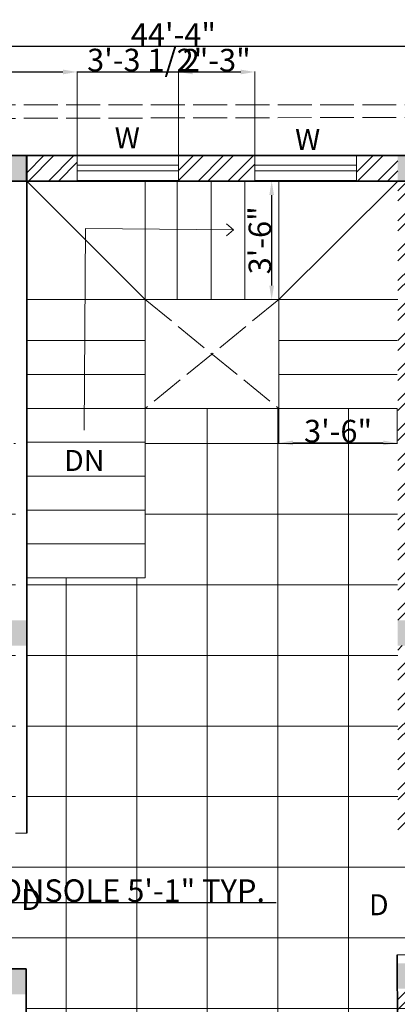
# Model space of a CAD drawing. Units: inches. Extents: x 351 to 1738, y -265 to 286.
# Tile 28 of 38: x 1246 to 1380, y -63 to 286. Entities that reach past the tile are written whole.
import ezdxf

# ---------------------------------------------------------------- set-up
doc = ezdxf.new("R2010")
doc.units = ezdxf.units.IN
doc.header["$MEASUREMENT"] = 0
doc.linetypes.add('ACAD_ISO02W100', pattern=[15, 12, -3])
for name, color, linetype, lineweight in [('A-ANNO-DIMS', 2, 'Continuous', 18), ('A-ANNO-SYMB', 7, 'Continuous', 18), ('A-COLS', 7, 'Continuous', 40), ('A-COLS-PATT', 6, 'Continuous', 13), ('A-DOOR', 3, 'Continuous', 18), ('A-FLOR-OVHD', 1, 'ACAD_ISO02W100', 18), ('A-FLOR-PATT', 9, 'Continuous', 9), ('A-FLOR-STRS', 7, 'Continuous', 18), ('A-FLOR-STRS-HIDN', 7, 'ACAD_ISO02W100', 13), ('A-GLAZ', 4, 'Continuous', 18), ('A-WALL', 7, 'Continuous', 35), ('A-WALL-PATT', 152, 'Continuous', 13)]:
    doc.layers.add(name, color=color, linetype=linetype, lineweight=lineweight)
doc.styles.add('Annotative', font='arial.ttf')
doc.styles.get("Standard").update_dxf_attribs({"font": 'arial.ttf'})
doc.dimstyles.get("Standard").update_dxf_attribs({"dimtxt": 8, "dimasz": 5, "dimexe": 0.18, "dimexo": 0.0625, "dimgap": 0.09, "dimtad": 1, "dimtoh": 1, "dimzin": 0, "dimdsep": 46, "dimlunit": 4, "dimtxsty": 'Standard', "dimcen": 0, "dimclre": 256, "dimadec": 0, "dimazin": 0, "dimtfac": 1, "dimtofl": 0, "dimtmove": 0, "dimatfit": 3, "dimfxl": 1, "dimtolj": 1, "dimtzin": 0, "dimlwe": -1, "dimarcsym": 0})

# ---------------------------------------------------------------- blocks, each defined once
blk = doc.blocks.new('*D7')
at = {"layer": 'A-ANNO-DIMS', "color": 0, "transparency": 16777216}
for p, q in [((1034.7, 256.03), (1034.7, 276.92)), ((1566.7, 256.03), (1566.7, 276.92))]:
    blk.add_line(p, q, dxfattribs=at)
at = {"layer": 'A-ANNO-DIMS', "color": 0, "lineweight": -2, "transparency": 16777216}
blk.add_line((1039.7, 276.74), (1561.7, 276.74), dxfattribs=at)
at = {"layer": 'A-ANNO-DIMS', "color": 0, "transparency": 16777216}
for points in [[(1039.7, 277.57), (1039.7, 275.91), (1034.7, 276.74)], [(1561.7, 277.57), (1561.7, 275.91), (1566.7, 276.74)]]:
    blk.add_solid(points, dxfattribs=at)
at = {"layer": 'Defpoints', "color": 0, "transparency": 16777216}
for p in [(1566.7, 276.74), (1034.7, 255.96), (1566.7, 255.96)]:
    blk.add_point(p, dxfattribs=at)
at = {"layer": 'A-ANNO-DIMS', "color": 0, "transparency": 16777216, "insert": (1300.7, 280.83), "char_height": 8, "attachment_point": 5}
blk.add_mtext('\\A1;44\'-4"', dxfattribs=at)
blk = doc.blocks.new('*D13')
at = {"layer": 'A-ANNO-DIMS', "color": 0, "transparency": 16777216}
for p, q in [((1338.06, 148.4), (1338.06, 136.03)), ((1380.06, 148.4), (1380.06, 136.03))]:
    blk.add_line(p, q, dxfattribs=at)
at = {"layer": 'A-ANNO-DIMS', "color": 0, "lineweight": -2, "transparency": 16777216}
blk.add_line((1343.06, 136.21), (1375.06, 136.21), dxfattribs=at)
at = {"layer": 'A-ANNO-DIMS', "color": 0, "transparency": 16777216}
for points in [[(1343.06, 137.05), (1343.06, 135.38), (1338.06, 136.21)], [(1375.06, 137.05), (1375.06, 135.38), (1380.06, 136.21)]]:
    blk.add_solid(points, dxfattribs=at)
at = {"layer": 'Defpoints', "color": 0, "transparency": 16777216}
for p in [(1338.06, 148.46), (1380.06, 148.46), (1380.06, 136.21)]:
    blk.add_point(p, dxfattribs=at)
at = {"layer": 'A-ANNO-DIMS', "color": 0, "transparency": 16777216, "insert": (1359.06, 140.39), "char_height": 8, "attachment_point": 5}
blk.add_mtext('\\A1;3\'-6"', dxfattribs=at)
blk = doc.blocks.new('*D14')
at = {"layer": 'A-ANNO-DIMS', "color": 0, "transparency": 16777216}
for p, q in [((1338, 228.96), (1335.35, 228.96)), ((1338, 186.96), (1335.35, 186.96))]:
    blk.add_line(p, q, dxfattribs=at)
at = {"layer": 'A-ANNO-DIMS', "color": 0, "lineweight": -2, "transparency": 16777216}
blk.add_line((1335.53, 191.96), (1335.53, 223.96), dxfattribs=at)
at = {"layer": 'A-ANNO-DIMS', "color": 0, "transparency": 16777216}
for points in [[(1334.69, 223.96), (1336.36, 223.96), (1335.53, 228.96)], [(1334.69, 191.96), (1336.36, 191.96), (1335.53, 186.96)]]:
    blk.add_solid(points, dxfattribs=at)
at = {"layer": 'Defpoints', "color": 0, "transparency": 16777216}
for p in [(1335.53, 228.96), (1338.06, 228.96), (1338.06, 186.96)]:
    blk.add_point(p, dxfattribs=at)
at = {"layer": 'A-ANNO-DIMS', "color": 0, "transparency": 16777216, "insert": (1331.35, 207.96), "char_height": 8, "attachment_point": 5, "rotation": 90}
blk.add_mtext('\\A1;3\'-6"', dxfattribs=at)
blk = doc.blocks.new('WIN-36')
for p, q in [((0, 5.5), (36, 5.5)), ((0, 3.5), (36, 3.5))]:
    blk.add_line(p, q)
blk.add_lwpolyline([(0, 9), (36, 9), (36, 0), (0, 0)], close=True)
blk = doc.blocks.new('*D42')
at = {"layer": 'A-ANNO-DIMS', "transparency": 16777216}
for p, q in [((1146.8, -35.63), (1146.8, -26.36)), ((1207.8, -35.63), (1207.8, -26.36))]:
    blk.add_line(p, q, dxfattribs=at)
at = {"layer": 'A-ANNO-DIMS', "color": 0, "lineweight": -2, "transparency": 16777216}
for p, q in [((1151.8, -26.54), (1202.8, -26.54)), ((1207.8, -26.54), (1337.09, -26.54))]:
    blk.add_line(p, q, dxfattribs=at)
at = {"layer": 'A-ANNO-DIMS', "color": 0, "transparency": 16777216}
for points in [[(1151.8, -25.71), (1151.8, -27.37), (1146.8, -26.54)], [(1202.8, -25.71), (1202.8, -27.37), (1207.8, -26.54)]]:
    blk.add_solid(points, dxfattribs=at)
at = {"layer": 'Defpoints', "color": 0, "transparency": 16777216}
for p in [(1207.8, -26.54), (1146.8, -35.69), (1207.8, -35.69)]:
    blk.add_point(p, dxfattribs=at)
at = {"layer": 'A-ANNO-DIMS', "color": 0, "transparency": 16777216, "insert": (1274.95, -22.31), "char_height": 8, "attachment_point": 5}
blk.add_mtext('\\A1;TV CONSOLE 5\'-1" TYP.', dxfattribs=at)
blk = doc.blocks.new('*D63')
at = {"layer": 'A-ANNO-DIMS', "transparency": 16777216}
for p, q in [((1227.04, 238.18), (1227.04, 267.75)), ((1266.55, 238.18), (1266.55, 267.75))]:
    blk.add_line(p, q, dxfattribs=at)
at = {"layer": 'A-ANNO-DIMS', "color": 0, "lineweight": -2, "transparency": 16777216}
for p, q in [((1232.04, 267.57), (1261.55, 267.57)), ((1266.55, 267.57), (1311.63, 267.57))]:
    blk.add_line(p, q, dxfattribs=at)
at = {"layer": 'A-ANNO-DIMS', "color": 0, "transparency": 16777216}
for points in [[(1232.04, 268.4), (1232.04, 266.73), (1227.04, 267.57)], [(1261.55, 268.4), (1261.55, 266.73), (1266.55, 267.57)]]:
    blk.add_solid(points, dxfattribs=at)
at = {"layer": 'Defpoints', "color": 0, "transparency": 16777216}
for p in [(1266.55, 267.57), (1227.04, 238.12), (1266.55, 238.12)]:
    blk.add_point(p, dxfattribs=at)
at = {"layer": 'A-ANNO-DIMS', "color": 0, "transparency": 16777216, "insert": (1291.59, 271.79), "char_height": 8, "attachment_point": 5}
blk.add_mtext('\\A1;3\'-3 1/2"', dxfattribs=at)
blk = doc.blocks.new('*D64')
at = {"layer": 'A-ANNO-DIMS', "transparency": 16777216}
for p, q in [((1302.55, 238.18), (1302.55, 267.75)), ((1329.55, 238.18), (1329.55, 267.75))]:
    blk.add_line(p, q, dxfattribs=at)
at = {"layer": 'A-ANNO-DIMS', "color": 0, "lineweight": -2, "transparency": 16777216}
blk.add_line((1307.55, 267.57), (1324.55, 267.57), dxfattribs=at)
at = {"layer": 'A-ANNO-DIMS', "color": 0, "transparency": 16777216}
for points in [[(1307.55, 268.4), (1307.55, 266.73), (1302.55, 267.57)], [(1324.55, 268.4), (1324.55, 266.73), (1329.55, 267.57)]]:
    blk.add_solid(points, dxfattribs=at)
at = {"layer": 'Defpoints', "color": 0, "transparency": 16777216}
for p in [(1329.55, 267.57), (1302.55, 238.12), (1329.55, 238.12)]:
    blk.add_point(p, dxfattribs=at)
at = {"layer": 'A-ANNO-DIMS', "color": 0, "transparency": 16777216, "insert": (1316.05, 271.74), "char_height": 8, "attachment_point": 5}
blk.add_mtext('\\A1;2\'-3"', dxfattribs=at)

msp = doc.modelspace()

# ---------------------------------------------------------------- hatches: boundary and pattern name
at = {"layer": 'A-COLS-PATT'}
h = msp.add_hatch(color=256, dxfattribs=at)
h.dxf.hatch_style = 1
h.paths.add_polyline_path([(1112.704, 237.963), (1103.704, 237.963), (1103.704, 228.963), (1112.704, 228.963)])
h.paths.add_polyline_path([(1115.704, 237.963), (1112.704, 237.963), (1112.704, 228.963), (1115.704, 228.963)])
h.paths.add_polyline_path([(1043.704, 255.963), (1034.704, 255.963), (1034.704, 243.963), (1043.704, 243.963)])
h.paths.add_polyline_path([(1043.704, 210.963), (1034.704, 210.963), (1034.704, 198.963), (1043.704, 198.963)])
h.paths.add_polyline_path([(1043.704, -45.037), (1034.704, -45.037), (1034.704, -57.037), (1043.704, -57.037)])
h.paths.add_polyline_path([(1112.704, -45.037), (1103.704, -45.037), (1103.704, -57.037), (1112.704, -57.037)])
h.paths.add_polyline_path([(1112.704, -161.037), (1103.704, -161.037), (1103.704, -164.037), (1103.704, -173.037), (1112.704, -173.037)])
h.paths.add_polyline_path([(1043.704, -161.037), (1034.704, -161.037), (1034.704, -173.037), (1043.704, -173.037)])
h.paths.add_polyline_path([(1248.549, -164.037), (1236.549, -164.037), (1236.549, -173.037), (1248.549, -173.037)])
h.paths.add_polyline_path([(1248.549, -50), (1236.549, -50), (1236.549, -59), (1248.549, -59)])
h.paths.add_polyline_path([(1248.704, 73.463), (1244.704, 73.463), (1244.704, 64.463), (1248.704, 64.463)])
h.paths.add_polyline_path([(1244.704, 73.463), (1236.704, 73.463), (1236.704, 64.463), (1244.704, 64.463)])
h.paths.add_polyline_path([(1248.704, 237.963), (1236.704, 237.963), (1236.704, 228.963), (1248.704, 228.963)])
h.paths.add_polyline_path([(1392.204, 237.963), (1380.204, 237.963), (1380.204, 228.963), (1392.204, 228.963)])
h.paths.add_polyline_path([(1536.064, 237.963), (1524.064, 237.963), (1524.064, 228.963), (1536.064, 228.963)])
h.paths.add_polyline_path([(1536.064, 73.463), (1524.064, 73.463), (1524.064, 64.463), (1536.064, 64.463)])
h.paths.add_polyline_path([(1384.204, 73.463), (1380.204, 73.463), (1380.204, 64.463), (1384.204, 64.463)])
h.paths.add_polyline_path([(1392.064, 73.463), (1384.204, 73.463), (1384.204, 64.463), (1392.064, 64.463)])
h.paths.add_polyline_path([(1536.064, -53.037), (1524.064, -53.037), (1524.064, -57.037), (1536.064, -57.037)])
h.paths.add_polyline_path([(1536.064, -48.037), (1524.064, -48.037), (1524.064, -53.037), (1536.064, -53.037)])
h.paths.add_polyline_path([(1392.064, -48.037), (1380.064, -48.037), (1380.064, -56.5), (1380.065, -57.037), (1392.064, -57.037)])
h.paths.add_polyline_path([(1536.064, -164.037), (1524.064, -164.037), (1524.064, -173.037), (1536.064, -173.037)])
at = {"layer": 'A-FLOR-PATT', "transparency": 33554559}
h = msp.add_hatch(dxfattribs=at)
h.set_pattern_fill('ANSI37', color=256, scale=200, angle=135)
h.set_pattern_definition([(180, (1112.704, -164.037), (-2e-15, -25), []), (270, (1112.704, -164.037), (25, -5e-15), [])])
h.paths.add_polyline_path([(1380.064, 73.463), (1380.132, 148.463), (1338.064, 148.463), (1290.704, 148.463), (1290.704, 88.463), (1248.704, 88.463), (1248.704, -2.009), (1244.704, -2.009), (1244.704, 142.457), (1160.704, 142.457), (1160.704, 158.963), (1160.704, 170.137), (1160.704, 206.137), (1160.704, 228.963), (1112.704, 228.963), (1112.704, 209.963), (1112.704, 168.963), (1124.704, 168.963), (1124.704, 162.963), (1112.704, 162.963), (1112.704, 64.463), (1112.704, 60.463), (1112.704, 0.463), (1112.704, -48.026), (1146.804, -47.981), (1146.804, -35.691), (1207.804, -35.691), (1207.804, -47.902), (1236.542, -47.864), (1236.544, -50.009), (1248.5, -50.009), (1248.506, -102.915), (1248.512, -150.915), (1248.514, -164.037), (1248.549, -164.037), (1273.017, -164.037), (1273.017, -128.799), (1355.24, -128.799), (1355.24, -164.037), (1384.204, -164.037), (1384.204, -57.037), (1380.064, -57.037), (1380.064, -48.037), (1392.064, -48.037), (1392.064, -53.037), (1406.549, -53.037), (1406.549, -57.037), (1401.204, -57.037), (1401.204, -147.037), (1468.204, -147.037), (1468.204, -138.5), (1472.204, -138.5), (1472.204, -102.5), (1468.204, -102.5), (1468.204, -57.037), (1442.549, -57.037), (1442.549, -53.037), (1463.049, -53.037), (1463.049, -40.747), (1524.049, -40.747), (1524.049, -48.037), (1536.064, -48.037), (1536.064, -53.037), (1557.704, -53.037), (1557.704, 204.963), (1384.204, 204.963), (1384.204, 73.463), (1392.064, 73.463), (1392.064, 64.463), (1384.204, 64.463), (1384.204, -3.5), (1380.204, -3.537), (1380.204, 64.463), (1380.064, 64.463)])
h.paths.add_polyline_path([(1510.714, 86.458, -0.1039845), (1511.661, 85.595, 0.4704384), (1510.158, 87.614, 0.0961001)], flags=16)
h.paths.add_polyline_path([(1510.443, 100.266, 0.009798), (1504.693, 100.48, 0.0287898), (1504.6, 99.767, -0.1653311), (1505.519, 96.135, -0.1436014)], flags=16)
h.paths.add_polyline_path([(1487.201, 85.595, -0.1039845), (1488.148, 86.458, 0.0961001), (1488.704, 87.614, 0.4704384)], flags=0)
h.paths.add_polyline_path([(1495.052, 100.43), (1494.178, 100.43, -0.0264629), (1494.262, 99.774, -0.1442193)], flags=16)
h.paths.add_polyline_path([(1444.485, 86.458, -0.1039845), (1445.433, 85.595, 0.4704384), (1443.93, 87.614, 0.0961001)], flags=16)
h.paths.add_polyline_path([(1420.972, 85.595, -0.1039845), (1421.92, 86.458, 0.0961001), (1422.475, 87.614, 0.4704384)], flags=16)
h.paths.add_polyline_path([(1428.632, 100.335, 0.0010541), (1427.971, 100.309, -0.0215241), (1428.033, 99.774, -0.1143008)], flags=16)
h.paths.add_polyline_path([(1419.906, 143.708, 0.0249793), (1420.222, 157.526), (1421.573, 159.101), (1421.573, 175.369), (1391.393, 175.369), (1391.393, 200.519), (1542.294, 200.519), (1542.294, 175.369), (1512.028, 175.369, 0.0198653), (1511.521, 153.838, 0.0251335), (1512.758, 118.323, 0.0205529), (1512.942, 115.253), (1419.834, 115.253, -0.0004142), (1419.843, 124.798), (1413.059, 124.798), (1413.059, 84.437, -0.0618528), (1415.831, 80.45, -0.0930773), (1420.972, 85.595, -0.2675367), (1422.371, 84.732, 0.0851103), (1424.052, 84.616, -0.8853927), (1424.033, 84.851, -1.1258145), (1424.073, 84.366, -0.0879871), (1422.371, 84.732, -0.2675367), (1422.326, 83.089, -0.3705421), (1420.972, 85.595, 0.0930773), (1415.831, 80.45, -0.0874142), (1417.914, 73.937), (1418.941, 73.937, 0.0272504), (1418.913, 76.906, -0.1157032), (1421.051, 73.937), (1445.354, 73.937, -0.1157032), (1447.492, 76.906, 0.0272504), (1447.464, 73.937), (1448.491, 73.937, -0.0874142), (1450.574, 80.45, 0.0930773), (1445.433, 85.595, -0.3705421), (1444.079, 83.089, -0.2675367), (1444.034, 84.732, -0.0879871), (1442.332, 84.366, -1.1258145), (1442.372, 84.851, -2.0327363), (1442.364, 84.368, 0.0863779), (1444.034, 84.732, -0.2675367), (1445.433, 85.595, -0.0930773), (1450.574, 80.45, -0.2577317), (1466.483, 90.927, -0.4786702), (1468.832, 91.907, -0.4786702), (1471.18, 90.927, -0.26264), (1483.053, 81.78, -0.0718662), (1487.201, 85.595, -0.2675367), (1488.6, 84.732, 0.0851103), (1490.28, 84.616, -0.8853927), (1490.262, 84.851, -1.1258145), (1490.301, 84.366, -0.0879871), (1488.6, 84.732, -0.2675367), (1488.554, 83.089, -0.3705421), (1487.201, 85.595, 0.0718662), (1483.053, 81.78, -0.1320648), (1484.143, 73.937), (1485.169, 73.937, 0.0272504), (1485.142, 76.906, -0.1157032), (1487.28, 73.937), (1511.582, 73.937, -0.1157032), (1513.72, 76.906, 0.0272504), (1513.693, 73.937), (1514.719, 73.937, -0.0874142), (1516.802, 80.45, 0.0930773), (1511.661, 85.595, -0.3705421), (1510.308, 83.089, -0.2675367), (1510.262, 84.732, -0.0879871), (1508.561, 84.366, -1.1258145), (1508.601, 84.851, -2.0327363), (1508.592, 84.368, 0.0863779), (1510.262, 84.732, -0.2675367), (1511.661, 85.595, -0.0930773), (1516.802, 80.45, -0.0618528), (1519.575, 84.437), (1519.575, 73.937), (1413.059, 73.937), (1413.059, 124.798), (1419.843, 124.798, -0.0008205)], flags=16)
h.paths.add_polyline_path([(1220.149, 54.133, -0.1039845), (1220.869, 53.476, 0.4704384), (1219.727, 55.011, 0.0961001)], flags=16)
h.paths.add_polyline_path([(1219.944, 64.626, 0.009798), (1215.574, 64.789, 0.0287898), (1215.503, 64.247, -0.1653311), (1216.201, 61.487, -0.1436014)], flags=16)
h.paths.add_polyline_path([(1209.779, 64.449, 0.0974459), (1209.339, 64.751), (1208.247, 64.751, 0.1273905), (1207.7, 64.326, 0.1715858), (1206.95, 61.475, -0.1588542), (1207.636, 59.45, 0.0158984), (1207.795, 59.218, 0.0615457), (1208.598, 59.616, 0.1754158), (1208.638, 60.099, -0.2847793), (1209.348, 62.472, 0.3262165)], flags=16)
h.paths.add_polyline_path([(1169.818, 54.133, -0.1039845), (1170.538, 53.476, 0.4704384), (1169.396, 55.011, 0.0961001)], flags=16)
h.paths.add_polyline_path([(1159.017, 62.472, 0.2847642), (1158.307, 60.099, -0.1754332), (1158.267, 59.616, 0.3929302), (1159.448, 64.449, -0.3262298)], flags=16)
h.paths.add_polyline_path([(1156.342, 58.239, -0.1783213), (1154.011, 55.31, -0.1747359), (1154.722, 55.233, -0.2008015), (1156.27, 56.086, 0.1269899), (1157.283, 58.991, -0.0912053)], flags=16)
h.paths.add_polyline_path([(1156.624, 61.413, 0.1572752), (1157.316, 64.247, 0.1696217)], flags=16)
h.paths.add_polyline_path([(1152.67, 54.133, -0.0961001), (1151.95, 53.476, 0.0640762), (1154.465, 54.384, 0.1990158)], flags=16)
h.paths.add_polyline_path([(1202.281, 53.476, -0.1039845), (1203, 54.133, 0.0961001), (1203.423, 55.011, 0.4704384)], flags=0)
h.paths.add_polyline_path([(1151.139, 97.64, 0.0249793), (1151.379, 108.141), (1152.406, 109.338), (1152.406, 121.701), (1129.47, 121.701), (1129.47, 140.814), (1244.149, 140.814), (1244.149, 121.701), (1221.148, 121.701, 0.0198653), (1220.763, 105.338, 0.0251335), (1221.703, 78.349, 0.0205529), (1221.843, 76.016), (1151.078, 76.016, -0.1287433), (1148.786, 65.037, 0.5393525), (1150.327, 64.171, -0.027594), (1163.481, 64.751, 0.0976954), (1163.04, 64.449, 0.3262165), (1163.471, 62.472, -0.2847765), (1164.181, 60.099, -0.1947567), (1165.846, 61.443, -0.1554021), (1165.172, 64.247, -0.1660224), (1165.869, 61.475, -0.1770142), (1167.852, 62.77, -0.4482027), (1169.974, 60.807, -0.3934987), (1167.679, 57.86, -0.8955483), (1168.438, 54.524, -0.3557668), (1166.218, 56.086, -0.066024), (1165.505, 57.539), (1165.251, 56.243, -0.3717324), (1164.02, 59.758, -0.3736141), (1163.04, 64.449, -0.0976954), (1163.481, 64.751, 0.0213538), (1153.294, 64.429, -0.1341826), (1156.695, 61.368, 0.1868727), (1154.636, 62.77, 0.4482027), (1152.514, 60.807, 0.4037263), (1154.905, 57.846, 0.7112192), (1153.334, 55, 0.5315397), (1151.95, 53.476, -0.2675367), (1153.013, 52.821, 0.0851103), (1154.29, 52.732, -0.8853927), (1154.276, 52.911, -1.1258145), (1154.306, 52.543, -0.0879871), (1153.013, 52.821, -0.2675367), (1152.978, 51.572, -0.3705421), (1151.95, 53.476, 0.0930773), (1148.043, 49.566, -0.0874142), (1149.626, 44.617), (1150.406, 44.617, 0.0272504), (1150.385, 46.873, -0.1157032), (1152.01, 44.617), (1170.478, 44.617, -0.1157032), (1172.103, 46.873, 0.0272504), (1172.082, 44.617), (1172.862, 44.617, -0.0874142), (1174.445, 49.566, 0.0930773), (1170.538, 53.476, -0.3705421), (1169.51, 51.572, -0.2675367), (1169.475, 52.821, -0.0879871), (1168.182, 52.543, -1.1258145), (1168.212, 52.911, -2.0327363), (1168.206, 52.544, 0.0863779), (1169.475, 52.821, -0.2675367), (1170.538, 53.476, -0.0930773), (1174.445, 49.566, -0.2577317), (1186.536, 57.528, -0.4786702), (1188.321, 58.273, -0.4786702), (1190.106, 57.528, -0.26264), (1199.128, 50.577, -0.0718662), (1202.281, 53.476, -0.2675367), (1203.344, 52.821, 0.0851103), (1204.621, 52.732, -0.8853927), (1204.607, 52.911, -1.1258145), (1204.637, 52.543, -0.0879871), (1203.344, 52.821, -0.2675367), (1203.309, 51.572, -0.3705421), (1202.281, 53.476, 0.0718662), (1199.128, 50.577, -0.1320648), (1199.957, 44.617), (1200.737, 44.617, 0.0272504), (1200.716, 46.873, -0.1157032), (1202.341, 44.617), (1220.809, 44.617, -0.1157032), (1222.434, 46.873, 0.0272504), (1222.413, 44.617), (1223.193, 44.617, -0.0874142), (1224.776, 49.566, 0.0930773), (1220.869, 53.476, -0.3705421), (1219.841, 51.572, -0.2675367), (1219.806, 52.821, -0.0879871), (1218.513, 52.543, -1.1258145), (1218.543, 52.911, -2.0327363), (1218.537, 52.544, 0.0863779), (1219.806, 52.821, -0.2675367), (1220.869, 53.476, -0.0930773), (1224.776, 49.566, -0.0618528), (1226.883, 52.597), (1226.883, 44.617), (1145.936, 44.617), (1145.936, 83.269), (1151.091, 83.269, -0.0008205)], flags=16)
h.paths.add_polyline_path([(1218.01, 57.86, -0.8955483), (1218.769, 54.524, -0.3557668), (1216.549, 56.086, -0.066024), (1215.836, 57.539), (1215.582, 56.243, -0.3717324), (1214.351, 59.758, -0.3736141), (1213.371, 64.449, 0.3262165), (1213.802, 62.472, -0.2847765), (1214.512, 60.099, -0.1947567), (1216.177, 61.443, -0.1799907), (1218.183, 62.77, -0.4482027), (1220.305, 60.807, -0.3934987)], flags=16)
h.paths.add_polyline_path([(1424.735, 91.363, -0.3934987), (1421.715, 95.241, -0.4482027), (1424.507, 97.824, -0.1799907), (1427.147, 96.077, -0.1947567), (1429.338, 94.309, -0.2847765), (1430.272, 97.432, 0.3262165), (1430.839, 100.034, -0.3736141), (1429.55, 93.861, -0.3717324), (1427.929, 89.235), (1427.596, 90.941, -0.066024), (1426.657, 89.029, -0.3557668), (1423.736, 86.973, -0.8955483)], flags=16)
h.paths.add_polyline_path([(1238.033, 131.257, -1), (1227.329, 131.257, -1)], flags=0)
h.paths.add_polyline_path([(1235.357, 131.257, -1), (1230.005, 131.257, -1)], flags=0)
h.paths.add_polyline_path([(1214.039, 54.243, 0.1543819), (1214.38, 53.992, 0.3589549), (1213.613, 54.016, 0.6039484), (1214.379, 53.657, 0.3713191), (1213.968, 52.872, 0.1879935), (1214.312, 52.809, -0.592455), (1213.953, 52.967, -0.2942791), (1214.083, 53.691, -1.3001871), (1213.881, 54.134, -0.2837621), (1214.469, 53.896, 1.1509396)], flags=16)
h.paths.add_polyline_path([(1212.091, 56.286, -0.4084338), (1211.337, 56.445, -0.0362594), (1211.098, 56.848, -0.2360976), (1211.59, 56.63, 0.0353445), (1211.835, 56.543, -0.4752408), (1212.091, 56.286, -0.4752408), (1212.438, 56.182, 0.0353445), (1212.631, 56.007, -0.2360976), (1213.056, 55.676, -0.0362594), (1212.588, 55.697, -0.4084338)], flags=16)
h.paths.add_polyline_path([(1211.469, 50.297, 0.296043), (1210.47, 50.527, 0.310883), (1211.931, 50.148, 0.0212546)], flags=16)
h.paths.add_polyline_path([(1213.739, 51.818, -0.0362594), (1213.271, 51.838, -0.4084337), (1212.774, 52.427, -0.0947856), (1212.293, 50.703, 1.1504738), (1212.911, 50.232, 0.1662877), (1213.265, 50.68, -0.0252543), (1212.603, 50.13, 1.0879317), (1212.471, 49.407, 0.1662877), (1213.02, 49.251, -0.016128), (1212.567, 49.563, -0.286859), (1212.217, 49.638, 0.0221563), (1212.046, 50.055, -0.6461302), (1212.185, 50.498, 0.0884116), (1212.732, 52.077, -1.1860374), (1213.121, 52.323, 0.0353445), (1213.314, 52.148, -0.2360976)], flags=16)
h.paths.add_polyline_path([(1212.094, 50.342, -0.0485241), (1211.54, 49.605, -1.1038339), (1211.397, 48.738, -0.7855147), (1211.683, 48.254, -0.3920429), (1210.948, 48.525, -0.3928194), (1210.561, 47.995, -0.592455), (1210.201, 48.153, -0.2942791), (1210.331, 48.877, -0.7041716), (1210.316, 49.592, -0.6793441), (1210.729, 50.112, 0.5636764)], flags=16)
h.paths.add_polyline_path([(1211.274, 49.829, -0.1398258), (1210.745, 49.859, -0.2178785), (1210.948, 49.509, -0.4985724)], flags=0)
h.paths.add_polyline_path([(1433.426, 81.49, -0.181571), (1434.245, 81.788, -0.0080665), (1433.726, 82.205, 0.0455784), (1432.755, 81.242, 0.1790113)], flags=16)
h.paths.add_polyline_path([(1434.146, 81.009, -0.1324418), (1433.645, 80.771, 0.2590893), (1433.234, 80.471, -0.1802109), (1433.392, 80.805, -0.1699398), (1432.758, 81.109, 0.0326525), (1433.273, 80.474, -0.4933627), (1434.046, 80.146, -0.3904966)], flags=16)
h.paths.add_polyline_path([(1434.83, 80.047, -0.9475376), (1435.294, 79.576, -0.2991282), (1434.625, 79.404, -0.2704392), (1435.01, 78.591, -0.592455), (1434.537, 78.382, -0.3928194), (1434.027, 79.08, -0.3920429), (1433.06, 78.723, -0.3520423), (1433.003, 79.197, -0.1972159), (1433.75, 79.734, -0.7136405), (1434.447, 79.939, -0.2147903), (1434.819, 80.475, 0.4088333), (1435.075, 80.803, -0.2261519)], flags=16)
h.paths.add_polyline_path([(1432.67, 81.217, -0.4542182), (1431.897, 79.923, -0.4144105), (1431.301, 80.035, 0.0161291), (1431.897, 80.445, 0.2795702), (1432.073, 80.871, -0.2895037), (1431.103, 81.321, -0.4144105), (1430.978, 81.915, 0.0161296), (1431.586, 81.521, 0.341293), (1432.125, 81.583, -0.8131856)], flags=16)
h.paths.add_polyline_path([(1429.893, 86.381, -0.9475376), (1430.358, 85.91, -0.1731062), (1429.984, 85.712, -0.0388172), (1431.625, 84.214, -0.0879005), (1432.097, 88.549, -0.0497684), (1431.254, 88.49, -0.2360976), (1431.814, 88.925, 0.0353445), (1432.067, 89.155, -0.4752408), (1432.524, 89.291, -0.4752408), (1432.86, 89.63, 0.0353445), (1433.182, 89.744, -0.2360976), (1433.83, 90.032, -0.0362594), (1433.516, 89.502, -0.4084338), (1432.524, 89.291, -0.3124239), (1432.106, 88.58, 0.0885594), (1431.625, 84.214, -0.4084337), (1430.971, 83.439, -0.0362594), (1430.355, 83.412, -0.2360976), (1430.914, 83.847, 0.0353445), (1431.168, 84.078, -0.4752408), (1431.625, 84.214, 0.0388172), (1429.984, 85.712, -0.3217316), (1429.333, 86.048, -0.32743), (1429.883, 86.809, 0.4088333), (1430.138, 87.138, -0.2261519)], flags=16)
h.paths.add_polyline_path([(1211.206, 58.616, -0.9997836), (1211.336, 59.323, -0.6149935)], flags=16)
h.paths.add_polyline_path([(1210.288, 49.429, 0.1543819), (1210.629, 49.178, 0.3589549), (1209.861, 49.202, 0.6039484), (1210.627, 48.843, -0.5348247), (1210.806, 49.295, 0.7483464)], flags=16)
h.paths.add_polyline_path([(1209.589, 51.828, -0.0087906), (1209.775, 51.753, 0.1122315), (1209.466, 52.019, 1.4188509), (1209.014, 51.708, -0.4587257), (1208.651, 51.073, -0.592455), (1208.291, 51.232, -0.2942791), (1208.421, 51.955, -1.3001871), (1208.219, 52.398, -0.2260052), (1208.719, 52.257, -0.4755189), (1209.158, 52.369, -1.4554994), (1209.603, 52.664, 0.4213049), (1209.191, 52.262, -0.5912116), (1208.979, 51.796, 0.4973986), (1209.773, 51.333, 0.6493116)], flags=16)
h.paths.add_polyline_path([(1208.029, 52.041, 0.5446671), (1208.832, 52.045, 0.220132)], flags=0)
h.paths.add_polyline_path([(1210.438, 51.425, -0.2041997), (1210.277, 52.018, 0.2708262), (1209.915, 52.897, 0.3241145)], flags=0)
h.paths.add_polyline_path([(1209.668, 52.407, -0.60139), (1208.99, 52.221, -0.3949159), (1208.248, 52.83, -0.8367916), (1208.651, 53.017, -0.3384876), (1209.039, 52.571, 0.1941379), (1209.191, 52.262, 0.4139945), (1209.712, 52.475, 0.5177103), (1210.503, 51.416, 0.401922), (1209.493, 50.93, 0.2063956), (1209.516, 50.165, -0.3194629), (1210.417, 51.418, -0.466635)], flags=16)
h.paths.add_polyline_path([(1206.601, 56.086, -0.3557668), (1204.381, 54.524, -0.9211983), (1205.236, 57.846, 0.2065693), (1207.614, 58.991, -0.1269899)], flags=16)
h.paths.add_polyline_path([(1435.487, 82.816, 0.5277653), (1436.615, 83.361, 0.5085402), (1437.05, 82.433, 0.592455), (1437.524, 82.641, 0.3312448), (1436.963, 83.548, 0.3878632), (1437.808, 83.626, 0.5929544), (1437.618, 84.176, 0.2260158), (1436.961, 83.99, 0.3182053), (1437.588, 84.854, 0.6893744), (1437.05, 84.991, 0.3357648), (1436.539, 84.41, -0.1569934), (1436.404, 84.065, -0.4346112), (1436.961, 83.99, -0.2147903), (1437.333, 84.526, 0.4088333), (1437.588, 84.854, -0.2261519), (1437.343, 84.097, -0.9475376), (1437.808, 83.626, -0.2991282), (1437.139, 83.455, -0.2704392), (1437.524, 82.641, -0.592455), (1437.05, 82.433, -0.3928194), (1436.541, 83.13, -0.4396601), (1435.475, 82.794, -0.174614), (1435.942, 82.244, -0.2063956), (1435.912, 81.237, -0.2708262), (1435.125, 82.208, 0.2079765), (1434.686, 82.904, -0.1964955)], flags=16)
h.paths.add_polyline_path([(1435.386, 84.832, 0.270811), (1434.91, 83.676, -0.2042174), (1434.699, 82.895, 0.3241145)], flags=0)
h.paths.add_polyline_path([(1435.68, 84.18, -0.2176564), (1435.554, 83.304, -0.1767045), (1436.236, 83.778, -0.3730364)], flags=0)
h.paths.add_polyline_path([(1435.566, 100.034, 0.3262165), (1436.133, 97.432, -0.2847765), (1437.067, 94.309, -0.1947567), (1439.258, 96.077, -0.1554021), (1438.371, 99.767, -0.1660224), (1439.289, 96.12, -0.1770142), (1441.897, 97.824, -0.4482027), (1444.69, 95.241, -0.3934987), (1441.67, 91.363, -0.8955483), (1442.669, 86.973, -0.3557668), (1439.748, 89.029, -0.066024), (1438.809, 90.941), (1438.476, 89.235, -0.3717324), (1436.855, 93.861, -0.3736141)], flags=16)
h.paths.add_polyline_path([(1191.252, 49.507, -0.2740221), (1190.658, 48.409, 0.2675367), (1191.311, 47.344, 0.3705421)], flags=0)
h.paths.add_polyline_path([(1190.301, 49.717, 0.1990158), (1188.619, 49.04, 0.0640762), (1191.252, 49.507, -0.0961001)], flags=0)
h.paths.add_polyline_path([(1189.518, 47.857, 1.1258145), (1189.676, 47.523, 2.0446052)], flags=0)
h.paths.add_polyline_path([(1464.974, 80.372, 0.2740221), (1465.756, 78.927, -0.0830131)], flags=0)
h.paths.add_polyline_path([(1464.974, 80.372, 0.3705421), (1464.897, 77.525, 0.5763244)], flags=0)
h.paths.add_polyline_path([(1464.974, 80.372, -0.4704384), (1467.284, 81.372, -0.0961001), (1466.226, 80.648, -0.1990158), (1468.439, 79.757, -0.0640762)], flags=0)
h.paths.add_polyline_path([(1189.511, 56.43, -0.2594668), (1188.321, 56.391, -0.2594668), (1187.13, 56.43, 0.0851103), (1188.193, 55.716, -0.8853927), (1188.27, 55.878, -1.1960133), (1188.355, 55.442, 0.1014587)], flags=0)
h.paths.add_polyline_path([(1188.321, 57.596, 0.0780722), (1187.678, 57.24, 0.0155503), (1188.321, 57.136, 0.0155503), (1188.964, 57.24, 0.0780722)], flags=0)
h.paths.add_polyline_path([(1190.164, 55.365, -0.5763244), (1190.106, 57.528, -0.1982945), (1188.321, 58.319, -0.1982945), (1186.536, 57.528, -0.5763244), (1186.477, 55.365, -0.3705421), (1186.536, 57.528, 0.1982945), (1188.321, 58.319, 0.1982945), (1190.106, 57.528, -0.3705421)], flags=0)
h.paths.add_polyline_path([(1188.372, 55.878, 1.1258145), (1188.529, 55.544, 2.0446052)], flags=0)
h.paths.add_polyline_path([(1186.341, 49.717, -0.0961001), (1185.389, 49.507, 0.0640762), (1188.022, 49.04, 0.1990158)], flags=0)
h.paths.add_polyline_path([(1185.389, 49.507, -0.2675367), (1185.984, 48.409, 0.0851103), (1187.046, 47.695, -0.8853927), (1187.123, 47.857, -1.1258145), (1186.966, 47.523, -0.0879871), (1185.984, 48.409, -0.2675367), (1185.331, 47.344, -0.3705421)], flags=0)
h.paths.add_polyline_path([(1399.441, 187.944, -1), (1413.525, 187.944, -1)], flags=0)
h.paths.add_polyline_path([(1402.962, 187.944, -1), (1410.004, 187.944, -1)], flags=0)
h.paths.add_polyline_path([(1357.663, -72.245), (1377.272, -72.245), (1377.272, -91.854), (1357.663, -91.854)], flags=16)
h.paths.add_polyline_path([(1467.256, 78.201, -1.1258145), (1467.049, 77.761, -2.0446052)], flags=0)
h.paths.add_polyline_path([(1468.822, 88.714, 0.9411249), (1469.106, 88.316, 1.1371523), (1468.765, 88.755, 0.890986), (1468.99, 88.245, 0.0948283), (1470.398, 89.481, -0.2675367), (1471.18, 90.927, -0.0281232), (1469.678, 90.547, -0.0287737), (1469.948, 90.311, -0.0203267), (1468.832, 90.41, -0.0203267), (1467.716, 90.311, -0.0287737), (1467.986, 90.547, -0.0281232), (1466.483, 90.927, -0.2675367), (1467.265, 89.481, 0.0851103), (1468.663, 88.542, -1.2023159)], flags=0)
h.paths.add_polyline_path([(1178.25, 124.523, -0.1199286), (1165.65, 124.145, -0.1073492), (1159.133, 124.446, -0.1028906), (1159.132, 130.465, -0.0748968), (1158.993, 137.956, 0.002027), (1167.844, 137.479, -0.07553), (1180.337, 137.666, -0.0758613), (1186.502, 137.688, -0.1409896), (1186.272, 130.046, -0.0954805), (1186.729, 124.748, -0.10603)], flags=0)
h.paths.add_polyline_path([(1469.225, 79.757, -0.1990158), (1471.437, 80.648, -0.0961001), (1470.379, 81.372, -0.4704384), (1472.689, 80.372, -0.3705421), (1472.766, 77.525, -0.2675367), (1471.907, 78.927, -0.0879863), (1470.615, 77.761, -1.1258491), (1470.408, 78.201, -2.0327363), (1470.642, 77.778, 0.0863779), (1471.907, 78.927, -0.2675367), (1472.689, 80.372, -0.0640762)], flags=0)
h.paths.add_polyline_path([(1430.423, 186.902, -0.0748968), (1430.24, 196.758, 0.002027), (1441.887, 196.131, -0.07553), (1458.326, 196.377, -0.0758613), (1466.438, 196.406, -0.1409896), (1466.136, 186.35, -0.0954805), (1466.737, 179.378, -0.10603), (1455.58, 179.082, -0.1199286), (1439, 178.585, -0.1073492), (1430.425, 178.981, -0.1028906)], flags=0)
h.paths.add_polyline_path([(1162.258, 49.939, 0.3357645), (1161.87, 49.497, -0.1569936), (1161.767, 49.235, -0.4346112), (1162.19, 49.178, -0.2147903), (1162.473, 49.585, 1.5291948)], flags=16)
h.paths.add_polyline_path([(1161.683, 49.021, 0.5815181), (1161.268, 49.583, 0.5927609)], flags=16)
h.paths.add_polyline_path([(1162.602, 48.058, 0.3713191), (1162.192, 48.843, 0.4345332), (1162.88, 48.962, 0.1850806), (1162.197, 48.926, 1.1218369)], flags=16)
h.paths.add_polyline_path([(1161.443, 48.941, -1.3071038), (1161.495, 48.571, -0.2177521), (1161.136, 48.254, 0.6973029), (1161.871, 49.048, 0.1215141)], flags=16)
h.paths.add_polyline_path([(1162.531, 49.429, -0.2070837), (1162.05, 49.146, -0.9920299)], flags=16)
h.paths.add_polyline_path([(1161.304, 49.578, -0.7196675), (1161.513, 50.079, -0.1304275), (1160.836, 50.168, 0.0395926)], flags=0)
h.paths.add_polyline_path([(1162.036, 50.584, -0.0080665), (1161.642, 50.9, 0.0293675), (1161.35, 50.297, -0.2057884)], flags=16)
h.paths.add_polyline_path([(1162.882, 51.392, -0.1247327), (1162.763, 51.828, -0.1011907), (1162.399, 51.438, -0.153425)], flags=0)
h.paths.add_polyline_path([(1164.235, 51.85, -0.3091075), (1164.513, 51.136, -0.6271245), (1163.781, 51.603, -0.6859091), (1162.777, 51.219, -0.2332851), (1163.303, 50.165, -0.2708262), (1162.705, 50.903, 0.2041997), (1162.381, 51.425, 0.204182), (1162.542, 52.018, -0.2708414), (1162.903, 52.897, -0.1272607), (1163.219, 52.529, -1.1686811), (1163.781, 52.587, -0.3291117), (1164.168, 53.017, -0.8367917), (1164.571, 52.83, -0.1933406), (1164.391, 52.338, -0.9475376), (1164.744, 51.981, -0.2991282)], flags=16)
h.paths.add_polyline_path([(1163.598, 51.937, -1.2629561), (1163.236, 51.831, 0.0125754), (1162.971, 51.721, 0.2306566), (1163.151, 52.407, -0.1648982), (1163.178, 52.661, -0.4493201), (1163.628, 52.262, -0.721477), (1164.154, 52.088, -0.8499982)], flags=0)
h.paths.add_polyline_path([(1161.613, 58.616, -0.9804131), (1161.525, 59.049, -2.9089348)], flags=16)
h.paths.add_polyline_path([(1160.252, 49.166, -0.4144105), (1159.799, 49.251, 0.0161291), (1160.252, 49.563, 0.2795702), (1160.386, 49.887, -0.2895037), (1159.649, 50.229, -0.4144105), (1159.554, 50.68, 0.0161296), (1160.015, 50.381, 0.6178854), (1160.526, 50.703, -0.0947856), (1160.045, 52.427, -0.1404436), (1159.682, 52.042, -0.0578559), (1159.3, 51.872, 0.5448433), (1160.046, 52.419, -0.0881216), (1160.404, 55.721, -0.0497684), (1159.763, 55.676, -0.2360976), (1160.188, 56.007, 0.0353445), (1160.381, 56.182, -0.4752408), (1160.728, 56.286, -0.4752408), (1160.984, 56.543, 0.0353445), (1161.229, 56.63, -0.2360976), (1161.721, 56.848, -0.0362594), (1161.482, 56.445, -0.4084338), (1160.728, 56.286, -0.3124239), (1160.411, 55.745, 0.0885594), (1160.045, 52.427, 0.1070813), (1160.634, 50.498, -0.4947977), (1160.839, 50.149, -0.4542182)], flags=16)
h.paths.add_polyline_path([(1160.666, 49.808, -2.0765276), (1160.828, 50.172, 0.0195861)], flags=0)
h.paths.add_polyline_path([(1158.439, 53.992, 0.1543819), (1158.78, 54.243, 0.7483463), (1158.262, 54.109, -0.3382251), (1158.492, 53.839, -0.1708158), (1159.124, 53.779, 0.4957286), (1158.938, 54.134, 0.2260157)], flags=16)
h.paths.add_polyline_path([(1160.045, 52.427, 0.0388172), (1158.798, 53.565, -0.1198178), (1158.574, 53.586, -0.3091075), (1158.851, 52.872, -0.1879935), (1158.506, 52.809, 0.592455), (1158.866, 52.967, 0.3312448), (1158.44, 53.657, 0.2012451), (1158.798, 53.565, -0.034023), (1159.901, 52.578, -0.0442527), (1159.698, 52.323, -0.4752408)], flags=16)
h.paths.add_polyline_path([(1336.926, -95.392), (1336.926, -117.945), (1291.82, -117.945), (1291.82, -95.392)], flags=16)
h.paths.add_polyline_path([(1357.535, -97.244), (1357.726, -96.697, 0.0348443)], flags=16)
h.paths.add_polyline_path([(1376.693, -96.478), (1377.301, -96.5, 0.0314968), (1375.907, -96.424), (1357.726, -96.424)], flags=16)
h.paths.add_polyline_path([(1379.403, -119.667, 0.0267056), (1380.043, -119.439, -0.0152991)], flags=16)
h.paths.add_polyline_path([(1357.726, -120.202), (1357.821, -120.202), (1357.821, -120.201)], flags=16)
h.paths.add_polyline_path([(1354.171, -104.592), (1354.469, -98.672, 0.0111377)], flags=16)
h.paths.add_polyline_path([(1355.058, -119.136), (1354.578, -118.539, 0.1431635)], flags=16)
h.paths.add_polyline_path([(1378.851, -96.821), (1378.85, -96.82), (1378.85, -96.82, -0.0496798), (1380.055, -97.191), (1378.85, -96.82, 0.1500541), (1375.135, -97.188), (1375.136, -119.44, -0.0099698), (1374.747, -116.649), (1357.726, -116.649, 0.1693849), (1357.535, -119.382), (1357.535, -119.382), (1357.535, -119.382, 0.0348176), (1357.726, -119.928), (1357.726, -119.928), (1357.726, -119.929, -0.0348772), (1357.535, -119.382), (1355.507, -119.382), (1355.317, -119.278), (1357.535, -119.382, -0.1693939), (1357.726, -116.649, -0.0391513), (1374.686, -116.113, -0.0020149), (1374.625, -115.546, 0.1153223), (1369.915, -115.474, 0.0609215), (1369.922, -101.154, 0.1151459), (1374.625, -101.079, -0.0020164), (1374.686, -100.513, -0.0391511), (1357.726, -99.977), (1374.747, -99.977, -0.0099633), (1375.135, -97.188), (1375.135, -97.188, -0.1501081)], flags=16)
h.paths.add_polyline_path([(1490.963, 91.363, -0.3934987), (1487.944, 95.241, -0.4482027), (1490.736, 97.824, -0.1799907), (1493.376, 96.077, -0.1947567), (1495.567, 94.309, -0.2847765), (1496.501, 97.432, 0.3262165), (1497.068, 100.034, -0.3736141), (1495.778, 93.861, -0.3717324), (1494.158, 89.235), (1493.824, 90.941, -0.066024), (1492.886, 89.029, -0.3557668), (1489.964, 86.973, -0.8955483)], flags=16)
h.paths.add_polyline_path([(1354.86, -97.658), (1355.316, -97.348, 0.1019112)], flags=16)
h.paths.add_polyline_path([(1497.063, 83.327, 0.1767244), (1496.37, 83.785, -0.4051388), (1496.016, 83.384, 0.4973986), (1497.06, 82.774, 0.6493116), (1496.818, 83.426, -0.0087906)], flags=16)
h.paths.add_polyline_path([(1496.339, 83.783, 0.5927609), (1496.886, 84.522, 0.5815181)], flags=16)
h.paths.add_polyline_path([(1495.11, 82.641, 0.592455), (1495.583, 82.433, 0.6769152), (1495.805, 83.59, 0.3756693)], flags=16)
h.paths.add_polyline_path([(1495.015, 84.176, -0.145057), (1495.301, 84.526, -0.4088333), (1495.045, 84.854, 0.2206292), (1495.381, 84.152, -0.199594), (1495.851, 83.764, -0.5240172), (1494.826, 83.626, -0.5929976)], flags=16)
h.paths.add_polyline_path([(1501.655, 81.915, -0.0161291), (1501.048, 81.521, -0.3927187), (1500.462, 81.37, -0.2106699), (1500.607, 81.142, 0.3066994)], flags=16)
h.paths.add_polyline_path([(1500.11, 89.291, -0.4084338), (1499.118, 89.502, -0.0362594), (1498.803, 90.032, -0.2360976), (1499.451, 89.744, 0.0353445), (1499.774, 89.63, -0.4752408), (1500.11, 89.291, -0.4752408), (1500.567, 89.155, 0.0353445), (1500.82, 88.925, -0.2360976), (1501.379, 88.49, -0.0362594), (1500.763, 88.516, -0.4084338)], flags=16)
h.paths.add_polyline_path([(1498.908, 82.205, -0.0513217), (1500.013, 81.134, -0.5879306), (1500.234, 81.676, 0.1070813), (1501.009, 84.214, -0.03529)], flags=16)
h.paths.add_polyline_path([(1496.93, 83.875, -0.2063956), (1497.247, 84.832, -0.2708262), (1497.724, 83.676, 0.2079765), (1497.944, 82.884, -0.3814554)], flags=16)
h.paths.add_polyline_path([(1496.721, 81.237, 0.2708125), (1497.509, 82.208, -0.2042157), (1497.935, 82.895, 0.3241145)], flags=16)
h.paths.add_polyline_path([(1497.529, 80.125, -0.145057), (1497.814, 80.475, -0.703182), (1498.282, 81.178, -0.1229248), (1497.977, 81.714, -0.2708368), (1499.207, 81.49, 0.2079641), (1499.993, 81.248, -0.2651454), (1499.278, 80.472, 0.3819006), (1498.808, 79.947, -0.3059049), (1498.848, 79.519, 0.4994816), (1498.574, 79.217, -0.4587257), (1498.097, 78.382, -0.592455), (1497.624, 78.591, -0.2704392), (1498.009, 79.404, -0.299116), (1497.34, 79.576, -0.5930157)], flags=16)
h.paths.add_polyline_path([(1500.736, 79.923, 0.4144105), (1501.333, 80.035, -0.3216484), (1500.192, 80.765, 0.0198856), (1499.976, 81.251, 0.4653307)], flags=16)
h.paths.add_polyline_path([(1501.009, 84.214, -0.0388172), (1502.649, 85.712, -0.1730946), (1502.276, 85.91, -0.5930157), (1502.465, 86.46, -0.145057), (1502.751, 86.809, -0.4088333), (1502.495, 87.138, 0.2206292), (1502.831, 86.436, -0.199594), (1503.301, 86.048, -0.3217316), (1502.649, 85.712, 0.0388172), (1501.009, 84.214, 0.1224486), (1501.412, 83.755, 0.4754908), (1501.335, 84.226, 0.055822), (1501.719, 83.847, -0.2360976), (1502.278, 83.412, -0.0362594), (1501.663, 83.439, -0.4084338)], flags=16)
h.paths.add_polyline_path([(1501.794, 100.034, 0.3262165), (1502.362, 97.432, -0.2847765), (1503.295, 94.309, -0.1947567), (1505.486, 96.077, -0.1799907), (1508.126, 97.824, -0.4482027), (1510.918, 95.241, -0.3934987), (1507.899, 91.363, -0.8955483), (1508.898, 86.973, -0.3557668), (1505.976, 89.029, -0.066024), (1505.038, 90.941), (1504.704, 89.235, -0.3717324), (1503.084, 93.861, -0.3736141)], flags=16)
h.paths.add_polyline_path([(1146.29, 131.257, -1), (1135.587, 131.257, -1)], flags=0)
h.paths.add_polyline_path([(1143.614, 131.257, -1), (1138.262, 131.257, -1)], flags=0)
h.paths.add_polyline_path([(1524.064, 73.463), (1536.064, 73.463), (1536.064, 64.463), (1524.064, 64.463)], flags=16)
h.paths.add_polyline_path([(1520.162, 187.944, -1), (1534.246, 187.944, -1)], flags=0)
h.paths.add_polyline_path([(1530.725, 187.944), (1527.204, 187.944), (1527.204, 184.423, 0.4142136)], flags=0)
h.paths.add_polyline_path([(1278.415, -91.154), (1331.067, -91.154), (1331.067, -80.583), (1278.415, -80.583)], flags=24)
h.paths.add_polyline_path([(1266.655, -79.354), (1354.738, -79.354), (1354.738, -67.817), (1266.655, -67.817)], flags=24)
h.paths.add_polyline_path([(1115.482, 206.184), (1155.098, 206.184), (1155.098, 217.714), (1115.482, 217.714)], flags=24)
h.paths.add_polyline_path([(1161.771, 8.501), (1222.466, 8.501), (1222.466, 19.079), (1161.771, 19.079)], flags=24)
h.paths.add_polyline_path([(1164.656, 18.795), (1210.615, 18.795), (1210.615, 30.324), (1164.656, 30.324)], flags=24)
h.paths.add_polyline_path([(1368.147, -32.882), (1379.362, -32.882), (1379.362, -21.733), (1368.147, -21.733)], flags=24)
h.paths.add_polyline_path([(1244.842, -31.012), (1256.057, -31.012), (1256.057, -19.863), (1244.842, -19.863)], flags=24)
h.paths.add_polyline_path([(1114.589, 195.739), (1156.517, 195.739), (1156.517, 206.31), (1114.589, 206.31)], flags=24)
h.paths.add_polyline_path([(1436.398, 37.632), (1505.131, 37.632), (1505.131, 48.203), (1436.398, 48.203)], flags=24)
h.paths.add_polyline_path([(1435.991, 47.919), (1507.906, 47.919), (1507.906, 59.456), (1435.991, 59.456)], flags=24)
h.paths.add_polyline_path([(1415.107, -124.896), (1457.038, -124.896), (1457.038, -114.318), (1415.107, -114.318)], flags=24)
h.paths.add_polyline_path([(1417.992, -114.602), (1457.609, -114.602), (1457.609, -103.073), (1417.992, -103.073)], flags=24)
at = {"layer": 'A-WALL-PATT'}
h = msp.add_hatch(dxfattribs=at)
h.set_pattern_fill('ANSI32', color=256, scale=20)
h.set_pattern_definition([(45, (1034.704, -173.037), (-5.3033, 5.3033), []), (45, (1038.24, -173.037), (-5.3033, 5.3033), [])])
h.paths.add_polyline_path([(1043.704, -57.037), (1034.704, -57.037), (1034.704, -81.037), (1043.704, -81.037)])
h.paths.add_polyline_path([(1043.704, 198.963), (1034.704, 198.963), (1034.704, -45.037), (1043.704, -45.037)])
h.paths.add_polyline_path([(1043.704, 243.963), (1034.704, 243.963), (1034.704, 237.963), (1034.704, 210.963), (1043.704, 210.963)])
h.paths.add_polyline_path([(1112.704, 255.963), (1043.704, 255.963), (1043.704, 246.963), (1103.704, 246.963), (1103.704, 237.963), (1112.704, 237.963), (1112.704, 251.963)])
h.paths.add_polyline_path([(1056.704, 207.963), (1043.704, 207.963), (1043.704, 198.963), (1056.704, 198.963)])
h.paths.add_polyline_path([(1103.704, 207.963), (1092.704, 207.963), (1092.704, 198.963), (1103.704, 198.963)])
h.paths.add_polyline_path([(1112.704, 228.963), (1103.704, 228.963), (1103.704, 74.963), (1112.704, 74.963), (1112.704, 97.5)])
h.paths.add_polyline_path([(1284.129, -164.037), (1248.549, -164.037), (1248.549, -173.037), (1284.129, -173.037)])
h.paths.add_polyline_path([(1524.064, -164.037), (1472.204, -164.037), (1472.204, -138.5), (1468.204, -138.5), (1468.204, -164.037), (1344.129, -164.037), (1344.129, -173.037), (1524.064, -173.037)])
h.paths.add_polyline_path([(1384.204, -57.037), (1380.065, -57.037), (1380.204, -164.037), (1384.204, -164.037)])
h.paths.add_polyline_path([(1566.704, -138), (1557.704, -138), (1557.704, -164.037), (1536.064, -164.037), (1536.064, -173.037), (1566.704, -173.037)])
h.paths.add_polyline_path([(1566.704, -30.189), (1557.704, -30.189), (1557.704, -53.037), (1536.064, -53.037), (1536.064, -57.037), (1557.704, -57.037), (1557.704, -102), (1566.704, -102)])
h.paths.add_polyline_path([(1524.064, -53.037), (1442.549, -53.037), (1442.549, -57.037), (1468.204, -57.037), (1468.204, -102.5), (1472.204, -102.5), (1472.204, -57.037), (1524.064, -57.037)])
h.paths.add_polyline_path([(1566.704, 120.993), (1557.704, 120.993), (1557.704, 29.811), (1566.704, 29.811)])
h.paths.add_polyline_path([(1384.204, 64.463), (1380.204, 64.463), (1380.204, -3.5), (1384.204, -3.5)])
h.paths.add_polyline_path([(1266.549, 237.963), (1248.704, 237.963), (1248.704, 228.963), (1266.549, 228.963)])
h.paths.add_polyline_path([(1329.549, 237.963), (1302.549, 237.963), (1302.549, 228.963), (1329.549, 228.963)])
h.paths.add_polyline_path([(1380.204, 237.963), (1365.549, 237.963), (1365.549, 228.963), (1380.204, 228.963)])
h.paths.add_polyline_path([(1524.064, 237.963), (1392.204, 237.963), (1392.204, 228.963), (1524.064, 228.963)])
h.paths.add_polyline_path([(1384.204, 228.963), (1380.204, 228.963), (1380.204, 73.463), (1384.204, 73.463)])
h.paths.add_polyline_path([(1566.704, 237.963), (1536.064, 237.963), (1536.064, 228.963), (1557.704, 228.963), (1557.704, 180.993), (1566.704, 180.993)])

# ---------------------------------------------------------------- linework, layer by layer
at = {"layer": 'A-ANNO-SYMB'}
for points in [[(1319.57, 209.541), (1321.972, 211.646), (1319.57, 213.751)], [(1269.071, 140.789), (1269.575, 212.141), (1321.972, 211.646)]]:
    msp.add_lwpolyline(points, dxfattribs=at)
at = {"layer": 'A-COLS'}
msp.add_lwpolyline([(1248.704, 228.963), (1248.704, 237.963)], dxfattribs=at)
at = {"layer": 'A-DOOR'}
for p, q in [((1248.704, -2.009), (1244.704, -2.009)), ((1384.204, -45), (1380.049, -45))]:
    msp.add_line(p, q, dxfattribs=at)
at = {"layer": 'A-FLOR-OVHD'}
for p, q in [((1112.704, 255.963), (1566.704, 255.963)), ((1112.704, 250.812), (1562.704, 251.963))]:
    msp.add_line(p, q, dxfattribs=at)
at = {"layer": 'A-FLOR-STRS'}
for p, q in [((1248.704, 228.963), (1290.704, 186.963)), ((1290.704, 88.463), (1290.704, 228.963)), ((1302.064, 186.963), (1302.064, 228.963)), ((1314.064, 186.963), (1314.064, 228.963)), ((1326.064, 186.963), (1326.064, 228.963)), ((1338.064, 148.463), (1338.064, 228.963)), ((1380.204, 228.963), (1338.064, 186.963)), ((1380.204, 186.963), (1248.704, 186.963)), ((1338.064, 148.463), (1338.064, 186.963)), ((1290.704, 172.463), (1248.704, 172.463)), ((1380.064, 172.463), (1338.064, 172.463)), ((1290.704, 160.463), (1248.704, 160.463)), ((1380.064, 160.463), (1338.064, 160.463)), ((1380.064, 148.463), (1248.704, 148.463)), ((1338.064, 148.463), (1289.417, 148.463)), ((1380.064, 148.463), (1338.064, 148.463)), ((1290.704, 136.463), (1248.704, 136.463)), ((1290.704, 124.463), (1248.704, 124.463)), ((1290.704, 112.463), (1248.704, 112.463)), ((1290.704, 100.463), (1248.704, 100.463)), ((1290.704, 88.463), (1248.704, 88.463))]:
    msp.add_line(p, q, dxfattribs=at)
at = {"layer": 'A-FLOR-STRS-HIDN'}
for p, q in [((1290.704, 186.963), (1338.064, 148.463)), ((1338.064, 186.963), (1290.704, 148.463))]:
    msp.add_line(p, q, dxfattribs=at)
at = {"layer": 'A-WALL'}
for p, q in [((1112.704, 237.963), (1248.704, 237.963)), ((1166.704, 228.963), (1248.704, 228.963)), ((1236.704, 228.963), (1557.704, 228.963)), ((1248.704, -2.009), (1248.704, 228.963)), ((1380.049, -45), (1380.204, -164.037)), ((1236.4, -50.009), (1248.5, -50.009)), ((1248.5, -50.009), (1248.506, -102.915))]:
    msp.add_line(p, q, dxfattribs=at)
msp.add_lwpolyline([(1566.704, 237.963), (1236.704, 237.963), (1236.704, 228.963)], dxfattribs=at)

# ---------------------------------------------------------------- block references
at = {"layer": 'A-GLAZ'}
for p in [(1266.549, 229.115), (1329.549, 229.115)]:
    msp.add_blockref('WIN-36', p, dxfattribs=at)

# ---------------------------------------------------------------- texts
at = {"layer": 'A-ANNO-SYMB', "style": 'Annotative'}
for s, height, p in [('W', 7.433, (1279.902, 240.499)), ('W', 7.433, (1343.836, 239.986)), ('DN', 7.4326, (1261.943, 126.289)), ('D', 7.433, (1246.7, -29.154)), ('D', 7.433, (1370.005, -31.024))]:
    msp.add_text(s, height=height, dxfattribs=at).set_placement(p)

# ---------------------------------------------------------------- dimensions: what is measured, and where the dimension line sits
at = {"layer": 'A-ANNO-DIMS'}
for base, p1, p2, override, picture, middle in [((1566.704, 276.74), (1034.704, 255.963), (1566.704, 255.963), {"dimclrd": 0, "dimclre": 0, "dimclrt": 0}, '*D7', (1300.704, 280.83)), ((1266.549, 267.565), (1227.038, 238.115), (1266.549, 238.115), {"dimdec": 1, "dimlfac": 1, "dimrnd": 0, "dimzin": 1, "dimdsep": 46, "dimlunit": 4, "dimfrac": 2}, '*D63', (1291.59, 271.794)), ((1329.549, 267.565), (1302.549, 238.115), (1329.549, 238.115), {"dimdec": 1, "dimlfac": 1, "dimrnd": 0, "dimzin": 1, "dimdsep": 46, "dimlunit": 4, "dimfrac": 2}, '*D64', (1316.049, 271.743)), ((1380.064, 136.213), (1338.064, 148.463), (1380.064, 148.463), {"dimclrd": 0, "dimclre": 0, "dimclrt": 0}, '*D13', (1359.064, 140.39))]:
    dim = msp.add_linear_dim(base=base, p1=p1, p2=p2, dimstyle='Standard', override=override, dxfattribs=at)
    dim.commit()
    dim.dimension.update_dxf_attribs({"geometry": picture, "text_midpoint": middle})
dim = msp.add_linear_dim(base=(1335.528, 228.963), p1=(1338.064, 186.963), p2=(1338.064, 228.963), angle=90, dimstyle='Standard', override={"dimclrd": 0, "dimclre": 0, "dimclrt": 0}, dxfattribs=at)
dim.commit()
dim.dimension.update_dxf_attribs({"geometry": '*D14', "text_midpoint": (1331.351, 207.963)})
dim = msp.add_linear_dim(base=(1207.804, -26.541), p1=(1146.804, -35.691), p2=(1207.804, -35.691), text='TV CONSOLE <> TYP.', dimstyle='Standard', override={"dimdec": 1, "dimlfac": 1, "dimrnd": 0, "dimzin": 1, "dimdsep": 46, "dimlunit": 4, "dimfrac": 2}, dxfattribs=at)
dim.commit()
dim.dimension.update_dxf_attribs({"geometry": '*D42', "text_midpoint": (1274.949, -22.312)})

doc.saveas('drawing.dxf')
